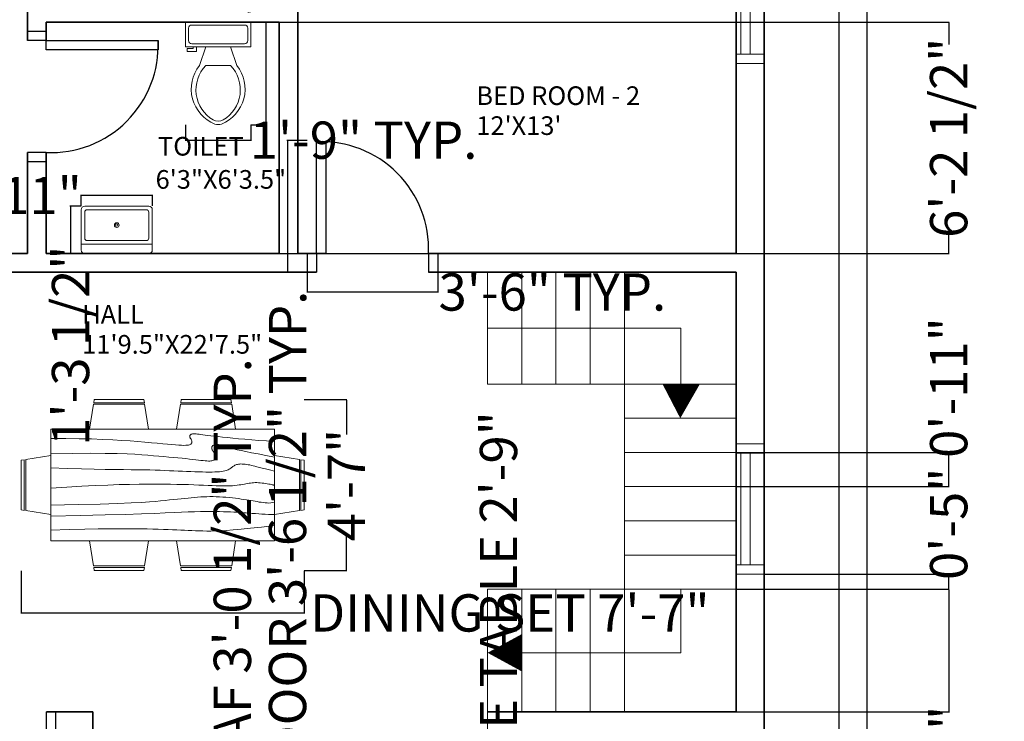
# Model space of a CAD drawing. Units: inches. Extents: x -107 to 531, y -526 to 131.
# Tile 3 of 4: x 205 to 522, y -340 to -114. Entities that reach past the tile are written whole.
import ezdxf

# ---------------------------------------------------------------- set-up
doc = ezdxf.new("R2010")
doc.units = ezdxf.units.IN
doc.header["$MEASUREMENT"] = 0
for name, color, linetype, lineweight in [('A-ANNO-DIMS', 2, 'Continuous', 18), ('A-AREA-IDEN', 7, 'Continuous', 25), ('A-DOOR', 3, 'Continuous', 25), ('A-FLOR-FIXT', 9, 'Continuous', 18), ('A-FLOR-STRS', 7, 'Continuous', 20), ('A-FURN', 8, 'Continuous', 18), ('A-GLAZ', 4, 'Continuous', 18), ('A-WALL', 7, 'Continuous', 35), ('C-PROP', 8, 'Continuous', 25)]:
    doc.layers.add(name, color=color, linetype=linetype, lineweight=lineweight)
doc.styles.get("Standard").update_dxf_attribs({"font": 'arial.ttf'})
doc.dimstyles.get("Standard").update_dxf_attribs({"dimtxt": 12, "dimasz": 0.18, "dimexe": 0.18, "dimexo": 0.0625, "dimgap": 0.09, "dimtad": 0, "dimdec": 1, "dimzin": 0, "dimdsep": 46, "dimlunit": 3, "dimtxsty": 'Standard', "dimcen": 0.09, "dimadec": 0, "dimazin": 0, "dimtfac": 1, "dimtdec": 1, "dimtofl": 0, "dimtmove": 0, "dimatfit": 3, "dimfxl": 1, "dimtolj": 1, "dimtzin": 0, "dimarcsym": 0})

# ---------------------------------------------------------------- blocks, each defined once
blk = doc.blocks.new('Toilet - top')
for p, q in [((9.5, -6), (9.5, -2)), ((-10, -8.5), (-8, -8.5)), ((-10, -9.5), (-10, -8.5)), ((-7, -9.5), (-10, -9.5)), ((-8, -8.5), (-8, -8)), ((-7, -8), (-7, -9.5)), ((-4, -8), (-6, -14)), ((4, -8), (6, -14)), ((4, -14), (-4, -14))]:
    blk.add_line(p, q)
blk.add_lwpolyline([(10.5, -8), (10.5, 0), (-10.5, 0), (-10.5, -8)], close=True)
for points in [[(-9.5, -2), (-9.5, -6)], [(8.5, -1), (-8.5, -1)], [(-8.5, -7), (8.5, -7)]]:
    blk.add_lwpolyline(points)
for centre, radius, start, end in [((-8.62, -1.88), 0.884, 81.8699, 188.1301), ((8.62, -1.88), 0.884, 351.8699, 98.1301), ((-8.62, -6.12), 0.884, 171.8699, 278.1301), ((8.62, -6.12), 0.884, 261.8699, 8.1301), ((3.52, -21.58), 12.17, 141.4691, 247.9714), ((4.2, -21.82), 11.33, 136.3677, 238.9468), ((-3.52, -21.58), 12.17, 292.0284, 38.5307), ((-4.2, -21.82), 11.33, 301.053, 43.6321), ((0, -27.88), 4, 245.7318, 294.2682), ((0, -29), 4, 254.8605, 285.1395)]:
    blk.add_arc(centre, radius, start, end)
blk = doc.blocks.new('Dining Set - 36 x 72 in.')
for p, q in [((-22.2343, 26.00059), (-23.4847, 17.99762)), ((-22.2304, 26), (-5.7608, 26)), ((-22, 27.5), (-22.1562, 26.50042)), ((-5.8416, 26.5), (-22.1534, 26.5)), ((-22, 27.5), (-6, 27.5)), ((-5.8437, 26.49966), (-6, 27.5)), ((-4.5152, 17.99762), (-5.7655, 25.99926)), ((5.7657, 26.00059), (4.5153, 17.99762)), ((5.7696, 26), (22.2392, 26)), ((6, 27.5), (5.8438, 26.50042)), ((22.1584, 26.5), (5.8466, 26.5)), ((6, 27.5), (22, 27.5)), ((22.1563, 26.49966), (22, 27.5)), ((23.4848, 17.99762), (22.2345, 25.99926)), ((36, 18), (-36, 18)), ((-36, 18), (-36, -18)), ((36, -18), (36, 18)), ((-45.5, 8), (-44.5004, 8.15617)), ((-45.5, 8), (-45.5, -8)), ((-44.5, -8.15843), (-44.5, 8.15338)), ((-44.0006, 8.23428), (-35.9976, 9.48474)), ((-44, 8.23041), (-44, -8.23915)), ((44.0006, 8.23428), (35.9976, 9.48474)), ((44, 8.23041), (44, -8.23915)), ((44.5, -8.15843), (44.5, 8.15338)), ((45.5, 8), (44.5005, 8.15617)), ((45.5, 8), (45.5, -8)), ((-44.4997, -8.15631), (-45.5, -8)), ((-35.9976, -9.48476), (-43.9993, -8.2345)), ((35.9976, -9.48476), (43.9993, -8.2345)), ((44.4997, -8.15631), (45.5, -8)), ((-36, -18), (36, -18)), ((-22.2343, -26.0006), (-23.4847, -17.99762)), ((-4.5152, -17.99762), (-5.7655, -25.99928)), ((5.7657, -26.0006), (4.5153, -17.99762)), ((23.4848, -17.99762), (22.2345, -25.99928)), ((-22.2304, -26), (-5.7608, -26)), ((-22, -27.5), (-22.1562, -26.50044)), ((-5.8416, -26.5), (-22.1534, -26.5)), ((-22, -27.5), (-6, -27.5)), ((-5.8437, -26.49967), (-6, -27.5)), ((5.7696, -26), (22.2392, -26)), ((6, -27.5), (5.8438, -26.50044)), ((22.1584, -26.5), (5.8466, -26.5)), ((6, -27.5), (22, -27.5)), ((22.1563, -26.49967), (22, -27.5))]:
    blk.add_line(p, q)
for points in [[(-36, 15), (-31.1772, 14.97754), (-26.8079, 14.91406), (-22.8538, 14.81543), (-19.276, 14.6875), (-16.0362, 14.53613), (-13.0957, 14.36718), (-10.4159, 14.18652), (-7.9583, 14), (-5.6904, 13.81315), (-3.6035, 13.63021), (-1.6954, 13.45508), (0.0365, 13.29166), (1.5945, 13.14388), (2.9811, 13.01562), (4.1988, 12.9108), (5.25, 12.83333), (6.1393, 12.78613), (6.8802, 12.76823), (7.4883, 12.77767), (7.9792, 12.8125), (8.3685, 12.87077), (8.6719, 12.95052), (8.9049, 13.0498), (9.0833, 13.16666), (9.2205, 13.29899), (9.3216, 13.44401), (9.3895, 13.59879), (9.4271, 13.76041), (9.4373, 13.92594), (9.4232, 14.09245), (9.3875, 14.257), (9.3333, 14.41666), (9.2638, 14.56917), (9.1836, 14.71484), (9.0975, 14.85465), (9.0104, 14.98958), (8.9272, 15.1206), (8.8529, 15.2487), (8.7922, 15.37483), (8.75, 15.5), (8.7305, 15.62467), (8.7344, 15.74739), (8.7617, 15.86621), (8.8125, 15.97916), (8.8867, 16.08431), (8.9844, 16.17968), (9.1055, 16.26334), (9.25, 16.33333), (9.4189, 16.38802), (9.6172, 16.42708), (9.8506, 16.45052), (10.125, 16.45833), (10.4463, 16.45052), (10.8203, 16.42708), (11.2529, 16.38802), (11.75, 16.33333), (12.3184, 16.26318), (12.9694, 16.17838), (13.7151, 16.07991), (14.5677, 15.96875), (15.5395, 15.84586), (16.6426, 15.71224), (17.8893, 15.56884), (19.2917, 15.41666), (20.859, 15.25667), (22.5879, 15.08984), (24.4721, 14.91715), (26.5052, 14.73958), (28.6809, 14.5581), (30.9929, 14.3737), (33.4347, 14.18733), (36, 14)], [(-36, 10), (-28.9766, 10.14274), (-23.1725, 10.20442), (-18.4241, 10.19775), (-14.5677, 10.13541), (-11.4399, 10.03011), (-8.877, 9.89453), (-6.7154, 9.74137), (-4.7917, 9.58333), (-2.9698, 9.43082), (-1.2246, 9.28515), (0.4415, 9.14534), (2.026, 9.01041), (3.5266, 8.87939), (4.9408, 8.7513), (6.266, 8.62516), (7.5, 8.5), (8.6411, 8.37549), (9.6914, 8.2539), (10.6538, 8.13818), (11.5312, 8.03125), (12.3267, 7.93603), (13.043, 7.85547), (13.6831, 7.79248), (14.25, 7.75), (14.7471, 7.7303), (15.1797, 7.73307), (15.5537, 7.75732), (15.875, 7.80208), (16.1494, 7.86637), (16.3828, 7.94922), (16.5811, 8.04964), (16.75, 8.16666), (16.8944, 8.29915), (17.0143, 8.44531), (17.1089, 8.60319), (17.1771, 8.77083), (17.218, 8.94629), (17.2305, 9.1276), (17.2137, 9.31282), (17.1667, 9.5), (17.0895, 9.6875), (16.987, 9.875), (16.8649, 10.0625), (16.7292, 10.25), (16.5856, 10.4375), (16.4401, 10.625), (16.2985, 10.8125), (16.1667, 11), (16.05, 11.18733), (15.9518, 11.3737), (15.8752, 11.5581), (15.8229, 11.73958), (15.798, 11.91715), (15.8034, 12.08984), (15.842, 12.25667), (15.9167, 12.41666), (16.0295, 12.56836), (16.1784, 12.70833), (16.3605, 12.83268), (16.5729, 12.9375), (16.8127, 13.01888), (17.0768, 13.07291), (17.3625, 13.0957), (17.6667, 13.08333), (17.9894, 13.03312), (18.3418, 12.94726), (18.7382, 12.82918), (19.1927, 12.68229), (19.7195, 12.51001), (20.3327, 12.31575), (21.0465, 12.10294), (21.875, 11.875), (22.8357, 11.63354), (23.959, 11.37304), (25.2786, 11.08618), (26.8282, 10.76562), (28.6414, 10.40405), (30.752, 9.99414), (33.1936, 9.52856), (36, 9)], [(-36, 5.5), (-30.7157, 5.3348), (-26.069, 5.20963), (-21.9946, 5.11767), (-18.4271, 5.05208), (-15.3009, 5.00602), (-12.5508, 4.97265), (-10.1112, 4.94515), (-7.9167, 4.91666), (-5.909, 4.88167), (-4.0586, 4.83984), (-2.3429, 4.79215), (-0.7396, 4.73958), (0.7739, 4.6831), (2.22, 4.6237), (3.6213, 4.56233), (5, 4.5), (6.373, 4.43782), (7.7344, 4.3776), (9.0723, 4.32129), (10.375, 4.27083), (11.6309, 4.22819), (12.8281, 4.19531), (13.9551, 4.17415), (15, 4.16666), (15.954, 4.17448), (16.819, 4.19791), (17.6001, 4.23698), (18.3021, 4.29166), (18.9299, 4.36198), (19.4883, 4.44791), (19.9823, 4.54948), (20.4167, 4.66666), (20.7969, 4.79899), (21.1302, 4.94401), (21.4245, 5.09879), (21.6875, 5.26041), (21.9271, 5.42594), (22.1511, 5.59245), (22.3672, 5.757), (22.5834, 5.91666), (22.8065, 6.06868), (23.0404, 6.21093), (23.2879, 6.34147), (23.5521, 6.45833), (23.8358, 6.55957), (24.142, 6.64323), (24.4735, 6.70735), (24.8334, 6.75), (25.2235, 6.76969), (25.642, 6.76692), (26.0858, 6.74267), (26.5521, 6.69791), (27.0379, 6.63362), (27.5404, 6.55078), (28.0565, 6.45036), (28.5834, 6.33333), (29.1242, 6.19987), (29.7071, 6.04687), (30.3661, 5.87044), (31.1354, 5.66666), (32.0493, 5.43164), (33.142, 5.16146), (34.4475, 4.85221), (36, 4.5)], [(-36, -1), (-30.7915, -0.6591), (-26.0195, -0.38216), (-21.6519, -0.16284), (-17.6563, 0.00521), (-14.0005, 0.12833), (-10.6523, 0.21289), (-7.5796, 0.26522), (-4.75, 0.29166), (-2.134, 0.29793), (0.2878, 0.28711), (2.5317, 0.26163), (4.6146, 0.22396), (6.5529, 0.17651), (8.3633, 0.12174), (10.0623, 0.06209), (11.6667, 0), (13.1899, -0.06201), (14.6341, -0.1211), (15.9982, -0.17432), (17.2813, -0.21875), (18.4823, -0.25147), (19.6003, -0.26953), (20.6343, -0.27002), (21.5834, -0.25), (22.4481, -0.20768), (23.2357, -0.14584), (23.9549, -0.06836), (24.6146, 0.02083), (25.2235, 0.11784), (25.7904, 0.21875), (26.3241, 0.31966), (26.8334, 0.41666), (27.3265, 0.50618), (27.8099, 0.58593), (28.2894, 0.65397), (28.7709, 0.70833), (29.2601, 0.74707), (29.763, 0.76823), (30.2855, 0.76985), (30.8334, 0.75), (31.4088, 0.70784), (31.9994, 0.64713), (32.589, 0.57275), (33.1615, 0.48958), (33.7008, 0.4025), (34.1908, 0.3164), (34.6153, 0.23616), (34.9584, 0.16666), (35.2099, 0.11165), (35.3848, 0.07031), (35.504, 0.04069), (35.5886, 0.02083), (35.6594, 0.00879), (35.7377, 0.0026), (35.8442, 0.00032), (36, 0)], [(-36, -6.5), (-27.1843, -6.31267), (-20.084, -6.1263), (-14.469, -5.9419), (-10.1094, -5.76042), (-6.7752, -5.58285), (-4.2363, -5.41016), (-2.2629, -5.24333), (-0.625, -5.08334), (0.8708, -4.93099), (2.2715, -4.78646), (3.5872, -4.64974), (4.8281, -4.52084), (6.0046, -4.39974), (7.127, -4.28646), (8.2053, -4.18099), (9.25, -4.08334), (10.2705, -3.99382), (11.2734, -3.91407), (12.2647, -3.84603), (13.25, -3.79167), (14.2354, -3.75293), (15.2266, -3.73177), (16.2295, -3.73015), (17.25, -3.75), (18.2912, -3.79248), (19.3451, -3.85547), (20.4009, -3.93604), (21.4479, -4.03125), (22.4754, -4.13819), (23.4727, -4.25391), (24.4289, -4.37549), (25.3334, -4.5), (26.1785, -4.62492), (26.9694, -4.74935), (27.7145, -4.87281), (28.4219, -4.99479), (29.1, -5.11483), (29.7572, -5.23242), (30.4016, -5.34709), (31.0417, -5.45834), (31.6837, -5.56437), (32.3262, -5.65821), (32.9658, -5.73153), (33.599, -5.77604), (34.2224, -5.78345), (34.8327, -5.74545), (35.4264, -5.65373), (36, -5.5)], [(-36, -10), (-26.4022, -9.81299), (-18.4675, -9.62891), (-11.9839, -9.45069), (-6.7396, -9.28125), (-2.5226, -9.12354), (0.8789, -8.98047), (3.6769, -8.85498), (6.0833, -8.75), (8.2767, -8.66765), (10.3021, -8.60677), (12.1712, -8.56543), (13.8958, -8.54167), (15.4876, -8.53353), (16.9583, -8.53907), (18.3197, -8.55632), (19.5834, -8.58334), (20.7616, -8.61841), (21.8685, -8.66081), (22.9188, -8.71004), (23.9271, -8.76563), (24.9081, -8.82707), (25.8763, -8.89388), (26.8465, -8.96558), (27.8334, -9.04167), (28.8474, -9.12118), (29.8828, -9.20117), (30.93, -9.27824), (31.9792, -9.34896), (33.0205, -9.40991), (34.0443, -9.45768), (35.0407, -9.48885), (36, -9.5)], [(-36, -14.5), (-30.0881, -14.33513), (-25.0332, -14.21224), (-20.7312, -14.12647), (-17.0781, -14.07292), (-13.97, -14.04671), (-11.3027, -14.04297), (-8.9724, -14.05681), (-6.875, -14.08334), (-4.9224, -14.11833), (-3.0905, -14.16016), (-1.3709, -14.20785), (0.2448, -14.26042), (1.7647, -14.3169), (3.1973, -14.3763), (4.5507, -14.43767), (5.8333, -14.5), (7.0554, -14.5621), (8.235, -14.62175), (9.3922, -14.67652), (10.5469, -14.72396), (11.7192, -14.76164), (12.929, -14.78711), (14.1965, -14.79794), (15.5417, -14.79167), (16.9933, -14.76424), (18.6152, -14.70508), (20.4804, -14.60197), (22.6615, -14.44271), (25.2312, -14.21509), (28.2624, -13.9069), (31.8277, -13.50594), (36, -13)]]:
    blk.add_lwpolyline(points)
blk = doc.blocks.new('Sink-single - 30 in top')
blk.add_line((-15, -3.999996), (15, -3.999996))
for points in [[(-13.5, 0), (13.5, 0)], [(-15, -18.499996), (-15, -1.5)], [(15, -1.5), (15, -18.499996)], [(-13.5, -17.499996), (-13.5, -6.499996)], [(-12.5, -5.499996), (12.5, -5.499996)], [(13.5, -6.499996), (13.5, -17.499996)], [(13.5, -19.999996), (-13.5, -19.999996)], [(12.5, -18.499996), (-12.5, -18.499996)]]:
    blk.add_lwpolyline(points)
for radius in [1, 0.5]:
    blk.add_circle((0, -11.999996), radius)
for centre, radius, start, end in [((-13.5, -1.5), 1.5, 90, 180), ((13.5, -1.5), 1.5, 0, 90), ((-12.5, -6.499996), 1, 90, 180), ((12.5, -6.499996), 1, 0, 90), ((-13.5, -18.499996), 1.5, 180, 270), ((-12.5, -17.499996), 1, 180, 270), ((12.5, -17.499996), 1, 270, 0), ((13.5, -18.499996), 1.5, 270, 0)]:
    blk.add_arc(centre, radius, start, end)
blk = doc.blocks.new('WIN-36')
for p, q in [((0, 0), (0, 9)), ((3, 0), (3, 9)), ((3, 9), (39, 9)), ((39, 7.5), (3, 7.5)), ((39, 9), (39, 0)), ((42, 9), (42, 0)), ((39, 4.5), (3, 4.5)), ((39, 0), (3, 0))]:
    blk.add_line(p, q)
blk = doc.blocks.new('DOOR-36-SWING')
for p, q in [((36.03, 42), (42.03, 42)), ((36.03, 39), (42.03, 39)), ((36.03, 3), (42.03, 3)), ((36.03, 0), (42.03, 0))]:
    blk.add_line(p, q)
blk.add_lwpolyline([(36.03, 3), (0.03, 3), (0.03, 6), (36.03, 6)], close=True)
blk.add_arc((34.53, 4.5), 34.53, 87.5104, 182.4896)
blk = doc.blocks.new('*D27')
at = {"layer": 'A-ANNO-DIMS', "color": 0, "lineweight": -2, "transparency": 16777216}
for p, q in [((268.43, -425.94), (274.01, -425.94)), ((273.83, -425.94), (273.83, -425.76)), ((273.83, -462.18), (273.83, -426.12)), ((268.43, -462.36), (274.01, -462.36))]:
    blk.add_line(p, q, dxfattribs=at)
at = {"layer": 'A-ANNO-DIMS', "color": 0, "transparency": 16777216}
for points in [[(273.8, -426.12), (273.86, -426.12), (273.83, -425.94)], [(273.8, -462.18), (273.86, -462.18), (273.83, -462.36)]]:
    blk.add_solid(points, dxfattribs=at)
at = {"layer": 'Defpoints', "color": 0, "transparency": 16777216}
for p in [(268.37, -425.94), (273.83, -425.94), (268.37, -462.36)]:
    blk.add_point(p, dxfattribs=at)
at = {"layer": 'A-ANNO-DIMS', "color": 0, "transparency": 16777216, "insert": (273.83, -321.4), "char_height": 12, "attachment_point": 5, "rotation": 90}
blk.add_mtext('\\A1;ENTRY LEAF 3\'-0 1/2" TYP.', dxfattribs=at)
blk = doc.blocks.new('*D29')
at = {"layer": 'A-ANNO-DIMS', "color": 0, "lineweight": -2, "transparency": 16777216}
for p, q in [((297.89, -152.94), (291.41, -152.94)), ((291.59, -153.12), (291.59, -195.18)), ((297.89, -195.36), (291.41, -195.36)), ((291.59, -195.36), (291.59, -195.54))]:
    blk.add_line(p, q, dxfattribs=at)
at = {"layer": 'A-ANNO-DIMS', "color": 0, "transparency": 16777216}
for points in [[(291.56, -153.12), (291.62, -153.12), (291.59, -152.94)], [(291.56, -195.18), (291.62, -195.18), (291.59, -195.36)]]:
    blk.add_solid(points, dxfattribs=at)
at = {"layer": 'Defpoints', "color": 0, "transparency": 16777216}
for p in [(297.95, -152.94), (291.59, -195.36), (297.95, -195.36)]:
    blk.add_point(p, dxfattribs=at)
at = {"layer": 'A-ANNO-DIMS', "color": 0, "transparency": 16777216, "insert": (291.59, -315.6), "char_height": 12, "attachment_point": 5, "rotation": 90}
blk.add_mtext('\\A1;INTERIOR DOOR 3\'-6 1/2" TYP.', dxfattribs=at)
blk = doc.blocks.new('*D30')
at = {"layer": 'A-ANNO-DIMS', "color": 0, "lineweight": -2, "transparency": 16777216}
for p, q in [((297.95, -195.42), (297.95, -201.9)), ((339.95, -195.42), (339.95, -201.9)), ((298.13, -201.72), (339.77, -201.72)), ((339.95, -201.72), (340.13, -201.72))]:
    blk.add_line(p, q, dxfattribs=at)
at = {"layer": 'A-ANNO-DIMS', "color": 0, "transparency": 16777216}
for points in [[(298.13, -201.69), (298.13, -201.75), (297.95, -201.72)], [(339.77, -201.69), (339.77, -201.75), (339.95, -201.72)]]:
    blk.add_solid(points, dxfattribs=at)
at = {"layer": 'Defpoints', "color": 0, "transparency": 16777216}
for p in [(297.95, -195.36), (339.95, -195.36), (339.95, -201.72)]:
    blk.add_point(p, dxfattribs=at)
at = {"layer": 'A-ANNO-DIMS', "color": 0, "transparency": 16777216, "insert": (376.79, -201.72), "char_height": 12, "attachment_point": 5}
blk.add_mtext('\\A1;3\'-6" TYP.', dxfattribs=at)
blk = doc.blocks.new('*D41')
at = {"layer": 'A-ANNO-DIMS', "color": 0, "lineweight": -2, "transparency": 16777216}
for p, q in [((225.21, -170.68), (225.03, -170.68)), ((225.21, -174.05), (225.21, -170.5)), ((247.92, -170.68), (225.39, -170.68)), ((248.1, -174.05), (248.1, -170.5))]:
    blk.add_line(p, q, dxfattribs=at)
at = {"layer": 'A-ANNO-DIMS', "color": 0, "transparency": 16777216}
for points in [[(225.39, -170.65), (225.39, -170.71), (225.21, -170.68)], [(247.92, -170.65), (247.92, -170.71), (248.1, -170.68)]]:
    blk.add_solid(points, dxfattribs=at)
at = {"layer": 'Defpoints', "color": 0, "transparency": 16777216}
for p in [(225.21, -170.68), (225.21, -174.11), (248.1, -174.11)]:
    blk.add_point(p, dxfattribs=at)
at = {"layer": 'A-ANNO-DIMS', "color": 0, "transparency": 16777216, "insert": (182.47, -170.68), "char_height": 12, "attachment_point": 5}
blk.add_mtext('\\A1;SINK 1\'-11"', dxfattribs=at)
blk = doc.blocks.new('*D42')
at = {"layer": 'A-ANNO-DIMS', "color": 0, "lineweight": -2, "transparency": 16777216}
for p, q in [((225.15, -174.11), (221.6, -174.11)), ((221.78, -174.29), (221.78, -189.18)), ((225.15, -189.36), (221.6, -189.36)), ((221.78, -189.36), (221.78, -189.54))]:
    blk.add_line(p, q, dxfattribs=at)
at = {"layer": 'A-ANNO-DIMS', "color": 0, "transparency": 16777216}
for points in [[(221.75, -174.29), (221.81, -174.29), (221.78, -174.11)], [(221.75, -189.18), (221.81, -189.18), (221.78, -189.36)]]:
    blk.add_solid(points, dxfattribs=at)
at = {"layer": 'Defpoints', "color": 0, "transparency": 16777216}
for p in [(225.21, -174.11), (221.78, -189.36), (225.21, -189.36)]:
    blk.add_point(p, dxfattribs=at)
at = {"layer": 'A-ANNO-DIMS', "color": 0, "transparency": 16777216, "insert": (221.78, -219), "char_height": 12, "attachment_point": 5, "rotation": 90}
blk.add_mtext('\\A1;1\'-3 1/2"', dxfattribs=at)
blk = doc.blocks.new('*D43')
at = {"layer": 'A-ANNO-DIMS', "color": 0, "lineweight": -2, "transparency": 16777216}
for p, q in [((279.83, -114.86), (284.9, -114.86)), ((284.72, -114.86), (284.72, -114.68)), ((284.72, -147.73), (284.72, -115.04)), ((279.83, -147.91), (284.9, -147.91))]:
    blk.add_line(p, q, dxfattribs=at)
at = {"layer": 'A-ANNO-DIMS', "color": 0, "transparency": 16777216}
for points in [[(284.69, -115.04), (284.75, -115.04), (284.72, -114.86)], [(284.69, -147.73), (284.75, -147.73), (284.72, -147.91)]]:
    blk.add_solid(points, dxfattribs=at)
at = {"layer": 'Defpoints', "color": 0, "transparency": 16777216}
for p in [(279.77, -114.86), (284.72, -114.86), (279.77, -147.91)]:
    blk.add_point(p, dxfattribs=at)
at = {"layer": 'A-ANNO-DIMS', "color": 0, "transparency": 16777216, "insert": (284.72, -61.48), "char_height": 12, "attachment_point": 5, "rotation": 90}
blk.add_mtext('\\A1;WC 2\'-9" TYP.', dxfattribs=at)
blk = doc.blocks.new('*D44')
at = {"layer": 'A-ANNO-DIMS', "color": 0, "lineweight": -2, "transparency": 16777216}
for p, q in [((258.77, -147.97), (258.77, -153.05)), ((279.77, -147.97), (279.77, -153.05)), ((258.95, -152.87), (279.59, -152.87)), ((279.77, -152.87), (279.95, -152.87))]:
    blk.add_line(p, q, dxfattribs=at)
at = {"layer": 'A-ANNO-DIMS', "color": 0, "transparency": 16777216}
for points in [[(258.95, -152.84), (258.95, -152.9), (258.77, -152.87)], [(279.59, -152.84), (279.59, -152.9), (279.77, -152.87)]]:
    blk.add_solid(points, dxfattribs=at)
at = {"layer": 'Defpoints', "color": 0, "transparency": 16777216}
for p in [(258.77, -147.91), (279.77, -147.91), (279.77, -152.87)]:
    blk.add_point(p, dxfattribs=at)
at = {"layer": 'A-ANNO-DIMS', "color": 0, "transparency": 16777216, "insert": (316.05, -152.87), "char_height": 12, "attachment_point": 5}
blk.add_mtext('\\A1;1\'-9" TYP.', dxfattribs=at)
blk = doc.blocks.new('*D49')
at = {"layer": 'A-ANNO-DIMS', "color": 0, "lineweight": -2, "transparency": 16777216}
for p, q in [((354.58, -397.68), (359.64, -397.68)), ((359.46, -397.68), (359.46, -397.5)), ((359.46, -430.49), (359.46, -397.86)), ((354.58, -430.67), (359.64, -430.67))]:
    blk.add_line(p, q, dxfattribs=at)
at = {"layer": 'A-ANNO-DIMS', "color": 0, "transparency": 16777216}
for points in [[(359.43, -397.86), (359.49, -397.86), (359.46, -397.68)], [(359.43, -430.49), (359.49, -430.49), (359.46, -430.67)]]:
    blk.add_solid(points, dxfattribs=at)
at = {"layer": 'Defpoints', "color": 0, "transparency": 16777216}
for p in [(354.51, -397.68), (359.46, -397.68), (354.51, -430.67)]:
    blk.add_point(p, dxfattribs=at)
at = {"layer": 'A-ANNO-DIMS', "color": 0, "transparency": 16777216, "insert": (359.46, -316.33), "char_height": 12, "attachment_point": 5, "rotation": 90}
blk.add_mtext('\\A1;COFFEE TABLE 2\'-9"', dxfattribs=at)
blk = doc.blocks.new('*D53')
at = {"layer": 'A-ANNO-DIMS', "color": 0, "lineweight": -2, "transparency": 16777216}
for p, q in [((205.89, -291.4), (205.89, -305.17)), ((296.89, -291.4), (296.89, -305.17)), ((206.07, -304.99), (296.71, -304.99)), ((296.89, -304.99), (297.07, -304.99))]:
    blk.add_line(p, q, dxfattribs=at)
at = {"layer": 'A-ANNO-DIMS', "color": 0, "transparency": 16777216}
for points in [[(206.07, -304.96), (206.07, -305.02), (205.89, -304.99)], [(296.71, -304.96), (296.71, -305.02), (296.89, -304.99)]]:
    blk.add_solid(points, dxfattribs=at)
at = {"layer": 'Defpoints', "color": 0, "transparency": 16777216}
for p in [(205.89, -291.34), (296.89, -291.34), (296.89, -304.99)]:
    blk.add_point(p, dxfattribs=at)
at = {"layer": 'A-ANNO-DIMS', "color": 0, "transparency": 16777216, "insert": (363.11, -304.99), "char_height": 12, "attachment_point": 5}
blk.add_mtext('\\A1;DINING SET 7\'-7"', dxfattribs=at)
blk = doc.blocks.new('*D54')
at = {"layer": 'A-ANNO-DIMS', "color": 0, "lineweight": -2, "transparency": 16777216}
for p, q in [((296.95, -236.34), (310.72, -236.34)), ((310.54, -236.52), (310.54, -247.56)), ((310.54, -291.16), (310.54, -280.12)), ((296.95, -291.34), (310.72, -291.34))]:
    blk.add_line(p, q, dxfattribs=at)
at = {"layer": 'A-ANNO-DIMS', "color": 0, "transparency": 16777216}
for points in [[(310.51, -236.52), (310.57, -236.52), (310.54, -236.34)], [(310.51, -291.16), (310.57, -291.16), (310.54, -291.34)]]:
    blk.add_solid(points, dxfattribs=at)
at = {"layer": 'Defpoints', "color": 0, "transparency": 16777216}
for p in [(296.89, -236.34), (310.54, -236.34), (296.89, -291.34)]:
    blk.add_point(p, dxfattribs=at)
at = {"layer": 'A-ANNO-DIMS', "color": 0, "transparency": 16777216, "insert": (310.54, -263.84), "char_height": 12, "attachment_point": 5, "rotation": 90}
blk.add_mtext('\\A1;4\'-7"', dxfattribs=at)
blk = doc.blocks.new('*D61')
at = {"layer": 'A-ANNO-DIMS', "color": 0, "lineweight": -2, "transparency": 16777216}
for p, q in [((436.01, -297.36), (504.48, -297.36)), ((504.3, -297.54), (504.3, -336.68)), ((436.01, -336.86), (504.48, -336.86)), ((504.3, -336.86), (504.3, -337.04))]:
    blk.add_line(p, q, dxfattribs=at)
at = {"layer": 'A-ANNO-DIMS', "color": 0, "transparency": 16777216}
for points in [[(504.27, -297.54), (504.33, -297.54), (504.3, -297.36)], [(504.27, -336.68), (504.33, -336.68), (504.3, -336.86)]]:
    blk.add_solid(points, dxfattribs=at)
at = {"layer": 'Defpoints', "color": 0, "transparency": 16777216}
for p in [(435.95, -297.36), (435.95, -336.86), (504.3, -336.86)]:
    blk.add_point(p, dxfattribs=at)
at = {"layer": 'A-ANNO-DIMS', "color": 0, "transparency": 16777216, "insert": (504.3, -367.06), "char_height": 12, "attachment_point": 5, "rotation": 90}
blk.add_mtext('\\A1;3\'-3 1/2"', dxfattribs=at)
blk = doc.blocks.new('*D62')
at = {"layer": 'A-ANNO-DIMS', "color": 0, "lineweight": -2, "transparency": 16777216}
for p, q in [((436.01, -253.36), (504.48, -253.36)), ((504.3, -253.36), (504.3, -253.18)), ((504.3, -264.18), (504.3, -253.54)), ((436.01, -264.36), (504.48, -264.36))]:
    blk.add_line(p, q, dxfattribs=at)
at = {"layer": 'A-ANNO-DIMS', "color": 0, "transparency": 16777216}
for points in [[(504.27, -253.54), (504.33, -253.54), (504.3, -253.36)], [(504.27, -264.18), (504.33, -264.18), (504.3, -264.36)]]:
    blk.add_solid(points, dxfattribs=at)
at = {"layer": 'Defpoints', "color": 0, "transparency": 16777216}
for p in [(435.95, -253.36), (504.3, -253.36), (435.95, -264.36)]:
    blk.add_point(p, dxfattribs=at)
at = {"layer": 'A-ANNO-DIMS', "color": 0, "transparency": 16777216, "insert": (504.3, -232.48), "char_height": 12, "attachment_point": 5, "rotation": 90}
blk.add_mtext('\\A1;0\'-11"', dxfattribs=at)
blk = doc.blocks.new('*D74')
at = {"layer": 'A-ANNO-DIMS', "color": 0, "lineweight": -2, "transparency": 16777216}
for p, q in [((445.01, -292.54), (504.48, -292.54)), ((504.3, -292.54), (504.3, -292.36)), ((504.3, -297.18), (504.3, -292.72)), ((436.01, -297.36), (504.48, -297.36))]:
    blk.add_line(p, q, dxfattribs=at)
at = {"layer": 'A-ANNO-DIMS', "color": 0, "transparency": 16777216}
for points in [[(504.27, -292.72), (504.33, -292.72), (504.3, -292.54)], [(504.27, -297.18), (504.33, -297.18), (504.3, -297.36)]]:
    blk.add_solid(points, dxfattribs=at)
at = {"layer": 'Defpoints', "color": 0, "transparency": 16777216}
for p in [(444.95, -292.54), (504.3, -292.54), (435.95, -297.36)]:
    blk.add_point(p, dxfattribs=at)
at = {"layer": 'A-ANNO-DIMS', "color": 0, "transparency": 16777216, "insert": (504.3, -276.32), "char_height": 12, "attachment_point": 5, "rotation": 90}
blk.add_mtext('\\A1;0\'-5"', dxfattribs=at)
blk = doc.blocks.new('*D76')
at = {"layer": 'A-ANNO-DIMS', "color": 0, "lineweight": -2, "transparency": 16777216}
for p, q in [((289.01, -114.86), (504.48, -114.86)), ((504.3, -115.04), (504.3, -122.06)), ((504.3, -189.18), (504.3, -182.17)), ((289.01, -189.36), (504.48, -189.36))]:
    blk.add_line(p, q, dxfattribs=at)
at = {"layer": 'A-ANNO-DIMS', "color": 0, "transparency": 16777216}
for points in [[(504.27, -115.04), (504.33, -115.04), (504.3, -114.86)], [(504.27, -189.18), (504.33, -189.18), (504.3, -189.36)]]:
    blk.add_solid(points, dxfattribs=at)
at = {"layer": 'Defpoints', "color": 0, "transparency": 16777216}
for p in [(288.95, -114.86), (504.3, -114.86), (288.95, -189.36)]:
    blk.add_point(p, dxfattribs=at)
at = {"layer": 'A-ANNO-DIMS', "color": 0, "transparency": 16777216, "insert": (504.3, -152.11), "char_height": 12, "attachment_point": 5, "rotation": 90}
blk.add_mtext('\\A1;6\'-2 1/2"', dxfattribs=at)

msp = doc.modelspace()

# ---------------------------------------------------------------- linework, layer by layer
at = {"layer": 'A-FLOR-STRS'}
for p, q in [((355.95, -195.36), (355.95, -231.36)), ((366.95, -195.36), (366.95, -231.36)), ((377.95, -195.36), (377.95, -231.36)), ((388.95, -195.36), (388.95, -231.36)), ((399.95, -195.36), (399.95, -336.86)), ((355.95, -231.36), (435.95, -231.36)), ((399.95, -242.36), (435.95, -242.36)), ((399.95, -253.36), (435.95, -253.36)), ((399.95, -264.36), (435.95, -264.36)), ((399.95, -275.36), (435.95, -275.36)), ((399.95, -286.36), (435.95, -286.36)), ((355.95, -297.36), (435.95, -297.36)), ((355.95, -297.36), (355.95, -342.86)), ((366.95, -297.36), (366.95, -336.86)), ((377.95, -297.36), (377.95, -336.86)), ((388.95, -297.36), (388.95, -336.86))]:
    msp.add_line(p, q, dxfattribs=at)
for points in [[(355.95, -213.36), (418.17, -213.36), (418.17, -231.36)], [(418.17, -297.36), (418.17, -317.81), (366.95, -317.81)]]:
    msp.add_lwpolyline(points, dxfattribs=at)
for points in [[(418.17, -231.36, 12, 0, 0), (417.95, -242.36, 0, 0, 0)], [(366.95, -317.81, 12, 0, 0), (355.95, -317.81, 0, 0, 0)]]:
    msp.add_lwpolyline(points, format="xyseb", dxfattribs=at)
at = {"layer": 'A-WALL'}
for p, q in [((444.95, -24.36), (444.95, -462.36)), ((207.95, -120.86), (207.95, -33.36)), ((435.95, -33.36), (435.95, -189.36)), ((294.95, -189.36), (294.95, -102.86)), ((213.95, -114.86), (288.95, -114.86)), ((213.95, -120.86), (213.95, -114.86)), ((288.95, -189.36), (288.95, -114.86)), ((207.95, -189.36), (207.95, -156.86)), ((213.95, -189.36), (213.95, -156.86)), ((201.95, -189.36), (207.95, -189.36)), ((213.95, -189.36), (288.95, -189.36)), ((294.95, -189.36), (300.95, -189.36)), ((336.95, -189.36), (435.95, -189.36)), ((201.95, -195.36), (300.95, -195.36)), ((336.95, -195.36), (435.95, -195.36)), ((435.95, -195.36), (435.95, -336.86)), ((214.07, -336.86), (228.95, -336.86)), ((228.95, -342.86), (228.95, -336.86)), ((355.95, -336.86), (435.95, -336.86))]:
    msp.add_line(p, q, dxfattribs=at)
at = {"layer": 'C-PROP'}
msp.add_line((468.95, -0.36), (468.95, -462.36), dxfattribs=at)
msp.add_lwpolyline([(231.95, -471.36), (21.95, -471.36), (21.95, 8.64), (477.95, 8.64), (477.95, -471.36), (303.95, -471.36)], dxfattribs=at)

# ---------------------------------------------------------------- block references
at = {"layer": 'A-DOOR'}
for p, rotation in [((249.98, -117.86), 180), ((297.95, -153.33), 270), ((217.07, -378.89), 89.99999999999991)]:
    msp.add_blockref('DOOR-36-SWING', p, dxfattribs=dict(at, rotation=rotation))
at = {"layer": 'A-FLOR-FIXT'}
msp.add_blockref('Toilet - top', (269.27, -114.86), dxfattribs=at)
at = {"layer": 'A-FLOR-FIXT', "xscale": 0.762708604536192, "yscale": 0.762708604536192, "zscale": 0.762708604536192, "rotation": 180}
msp.add_blockref('Sink-single - 30 in top', (236.65, -189.36), dxfattribs=at)
at = {"layer": 'A-FURN'}
msp.add_blockref('Dining Set - 36 x 72 in.', (251.39, -263.84), dxfattribs=at)
at = {"layer": 'A-GLAZ'}
for p, rotation in [((444.95, -128.17), 89.99999999999987), ((444.95, -292.54), 90.00000000000017)]:
    msp.add_blockref('WIN-36', p, dxfattribs=dict(at, rotation=rotation))

# ---------------------------------------------------------------- texts
at = {"layer": 'A-AREA-IDEN'}
for s, p in [('BED ROOM - 2', (352.32, -141.56)), ("12'X13'", (352.32, -151.2)), ('TOILET', (249.92, -157.84)), ('6\'3"X6\'3.5"', (249.15, -168.5)), ('HALL', (225.54, -211.93)), ('11\'9.5"X22\'7.5"', (225.54, -221.57))]:
    msp.add_text(s, height=6, dxfattribs=at).set_placement(p)

# ---------------------------------------------------------------- dimensions: what is measured, and where the dimension line sits
at = {"layer": 'A-ANNO-DIMS'}
for base, p1, p2, angle, text, picture, middle in [((284.7239, -114.8618), (279.7669, -147.9081), (279.7669, -114.8618), 90, 'WC <> TYP.', '*D43', (284.7239, -61.48)), ((225.21, -170.68), (248.1, -174.11), (225.21, -174.11), 180, 'SINK <>', '*D41', (182.47, -170.68)), ((291.59, -195.36), (297.95, -152.94), (297.95, -195.36), 270, 'INTERIOR DOOR <> TYP.', '*D29', (291.59, -315.6)), ((273.83, -425.94), (268.37, -462.36), (268.37, -425.94), 90, 'ENTRY LEAF <> TYP.', '*D27', (273.83, -321.4)), ((359.46, -397.68), (354.51, -430.67), (354.51, -397.68), 90, 'COFFEE TABLE <>', '*D49', (359.46, -316.33))]:
    dim = msp.add_linear_dim(base=base, p1=p1, p2=p2, angle=angle, text=text, dimstyle='Standard', override={"dimdec": 1, "dimlfac": 1, "dimrnd": 0, "dimzin": 1, "dimdsep": 46, "dimlunit": 4, "dimfrac": 2}, dxfattribs=at)
    dim.commit()
    dim.dimension.update_dxf_attribs({"geometry": picture, "text_midpoint": middle})
for base, p1, p2, angle, picture, middle in [((504.3, -114.86), (288.95, -189.36), (288.95, -114.86), 90, '*D76', (504.3, -152.11)), ((221.7818, -189.3618), (225.214, -174.1077), (225.214, -189.3618), 270, '*D42', (221.7818, -218.9975)), ((504.3, -253.36), (435.95, -264.36), (435.95, -253.36), 90, '*D62', (504.3, -232.48)), ((310.54, -236.34), (296.89, -291.34), (296.89, -236.34), 90, '*D54', (310.54, -263.84)), ((504.3, -292.54), (435.95, -297.36), (444.95, -292.54), 90, '*D74', (504.3, -276.32)), ((504.3, -336.86), (435.95, -297.36), (435.95, -336.86), 90, '*D61', (504.3, -367.06))]:
    dim = msp.add_linear_dim(base=base, p1=p1, p2=p2, angle=angle, dimstyle='Standard', override={"dimdec": 1, "dimlfac": 1, "dimrnd": 0, "dimzin": 1, "dimdsep": 46, "dimlunit": 4, "dimfrac": 2}, dxfattribs=at)
    dim.commit()
    dim.dimension.update_dxf_attribs({"geometry": picture, "text_midpoint": middle})
for base, p1, p2, text, picture, middle in [((279.77, -152.87), (258.77, -147.91), (279.77, -147.91), '<> TYP.', '*D44', (316.05, -152.87)), ((339.95, -201.72), (297.95, -195.36), (339.95, -195.36), '<> TYP.', '*D30', (376.79, -201.72)), ((296.89, -304.99), (205.89, -291.34), (296.89, -291.34), 'DINING SET <>', '*D53', (363.11, -304.99))]:
    dim = msp.add_linear_dim(base=base, p1=p1, p2=p2, text=text, dimstyle='Standard', override={"dimdec": 1, "dimlfac": 1, "dimrnd": 0, "dimzin": 1, "dimdsep": 46, "dimlunit": 4, "dimfrac": 2}, dxfattribs=at)
    dim.commit()
    dim.dimension.update_dxf_attribs({"geometry": picture, "text_midpoint": middle})

doc.saveas('drawing.dxf')
